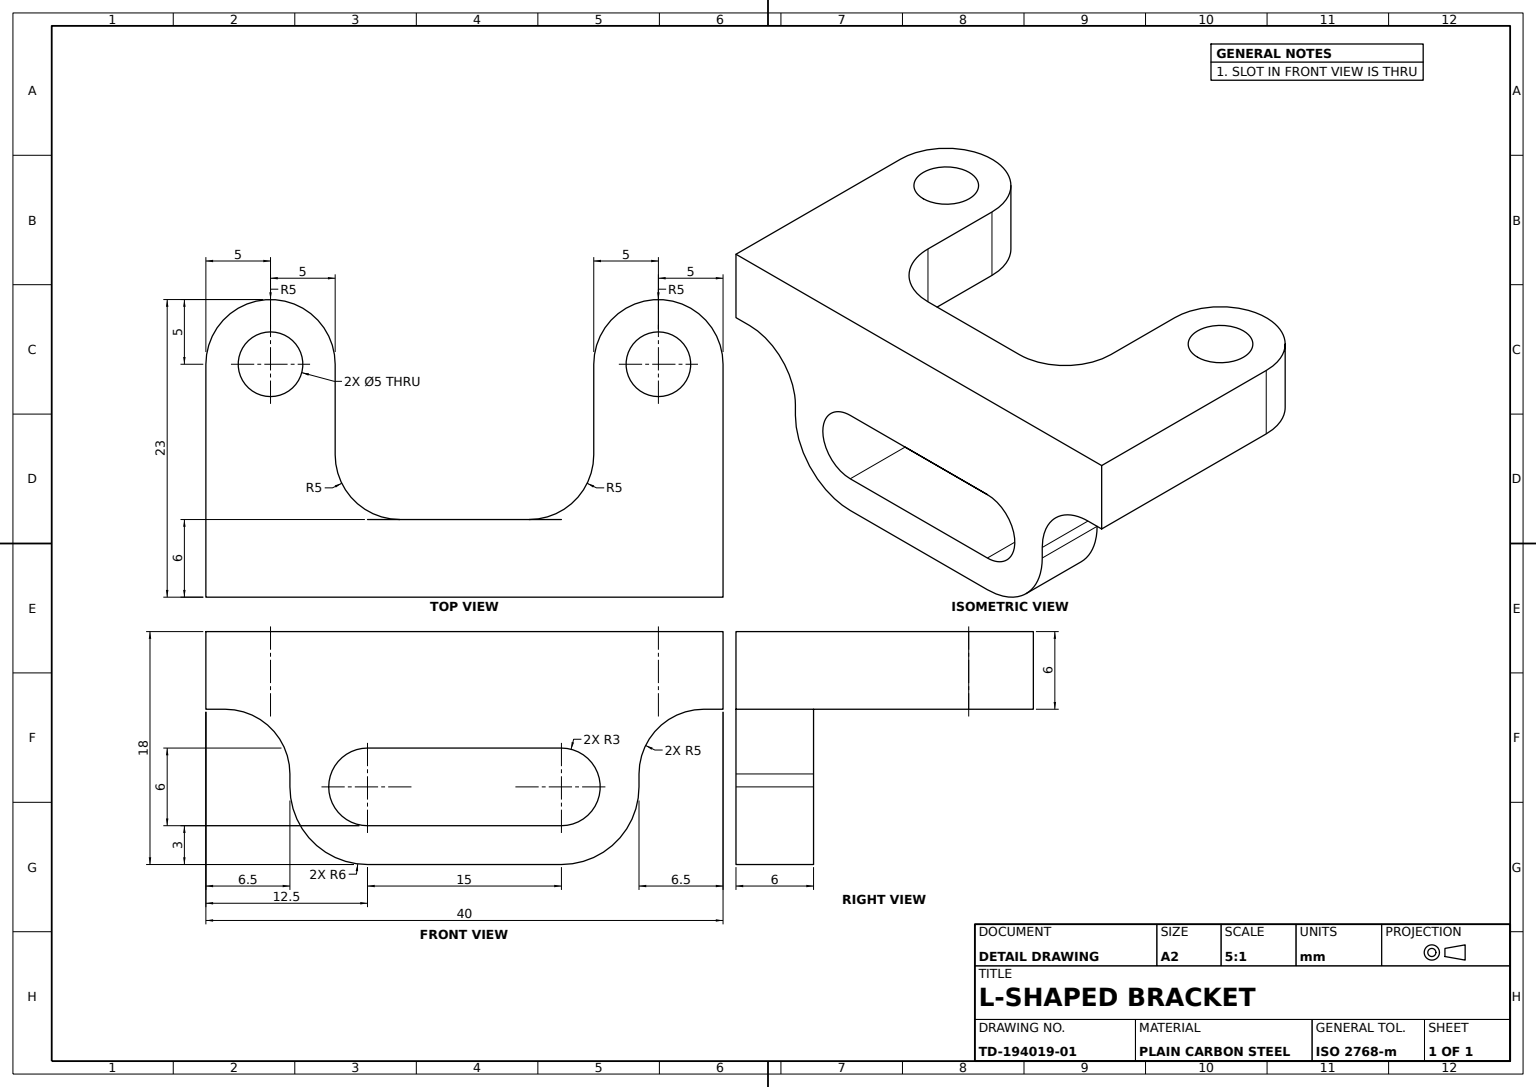
SolidWorks part; units mm, degrees
material "Plain Carbon Steel"
ref_plane "Front Plane" through (0, 0, 0) normal (0, 0, 1) x (1, 0, 0)
ref_plane "Top Plane" through (0, 0, 0) normal (0, 1, 0) x (1, 0, 0)
ref_plane "Right Plane" through (0, 0, 0) normal (1, 0, 0) x (0, 0, -1)
sketch "U Bracket Profile Sketch" plane through (0, 0, 0) normal (0, 0, 1) x (1, 0, 0)
  line L0 (0, 0) -> (40, 0)
  line L1 (40, 0) -> (40, -6)
  line L2 (0, 0) -> (0, -6)
  line L9 (6.5, -12) -> (6.5, -11)
  line L10 (33.5, -12) -> (33.5, -11)
  line L11 (12.5, -18) -> (27.5, -18)
  line L12 (0, -6) -> (1.5, -6)
  line L15 (40, -6) -> (38.5, -6)
  arc A2 (27.5, -18) -> (33.5, -12) centre (27.5, -12) ccw
  arc A3 (6.5, -12) -> (12.5, -18) centre (12.5, -12) ccw
  arc A4 (6.5, -11) -> (1.5, -6) centre (1.5, -11) ccw
  arc A5 (38.5, -6) -> (33.5, -11) centre (38.5, -11) ccw
  dimension "D1" = 5
  dimension "D2" = 5
  dimension "D5" = 5
  dimension "D6" = 6
  dimension "D9" = 6
  dimension "D3" = 18
  dimension "D4" = 6
  dimension "D7" = 12.5
  dimension "D8" = 40
  dimension "D10" = 12.5
extrude "U Bracket Base" add sketch "U Bracket Profile Sketch" along normal blind 6
sketch "Slotted Tab Sketch" plane through (0, 0, 0) normal (0, 1, 0) x (1, 0, 0)
  line L4 (0, 12) -> (0, 0)
  line L5 (40, 12) -> (40, 0)
  line L6 (0, 0) -> (15, 0)
  line L8 (25, 0) -> (40, 0)
  line L9 (10, 12) -> (10, 5)
  line L10 (30, 12) -> (30, 5)
  arc A0 (10, 12) -> (0, 12) centre (5, 12) ccw
  arc A1 (40, 12) -> (30, 12) centre (35, 12) ccw
  arc A2 (25, 0) -> (30, 5) centre (25, 5) ccw
  arc A3 (15, 0) -> (10, 5) centre (15, 5) cw
  point P0 (35, 17)
  dimension "D1" = 5
  dimension "D2" = 5
  dimension "D3" = 5
  dimension "D6" = 5
  dimension "D4" = 12
  dimension "D5" = 15
  dimension "D7" = 17
  dimension "D8" = 7
  dimension "D9" = 5
  dimension "D10" = 15
  dimension "D11" = 40
extrude "Slotted Tab" add sketch "Slotted Tab Sketch" against normal blind 6
sketch "Mounting Holes Sketch" plane through (0, -6, 0) normal (0, -1, 0) x (1, 0, 0)
  circle A0 centre (5, -12) radius 2.5
  circle A1 centre (35, -12) radius 2.5
  dimension "D1" = 5
extrude "Mounting Holes 2x" cut sketch "Mounting Holes Sketch" against normal blind 6
sketch "Tab Slot Sketch" plane through (0, 0, 0) normal (0, 0, -1) x (-1, 0, 0)
  line L0 (-15, -6) -> (-15, 0) construction
  line L1 (-25, 0) -> (-15, 0) construction
  line L4 (-27.5, -9) -> (-12.5, -9)
  line L6 (-12.5, -15) -> (-27.5, -15)
  arc A0 (-27.5, -9) -> (-27.5, -15) centre (-27.5, -12) ccw
  arc A1 (-12.5, -15) -> (-12.5, -9) centre (-12.5, -12) ccw
  dimension "D1" = 3
  dimension "D2" = 2.5
  dimension "D3" = 12.5
  dimension "D4" = 12
extrude "Tab Slot" cut sketch "Tab Slot Sketch" against normal blind 6
